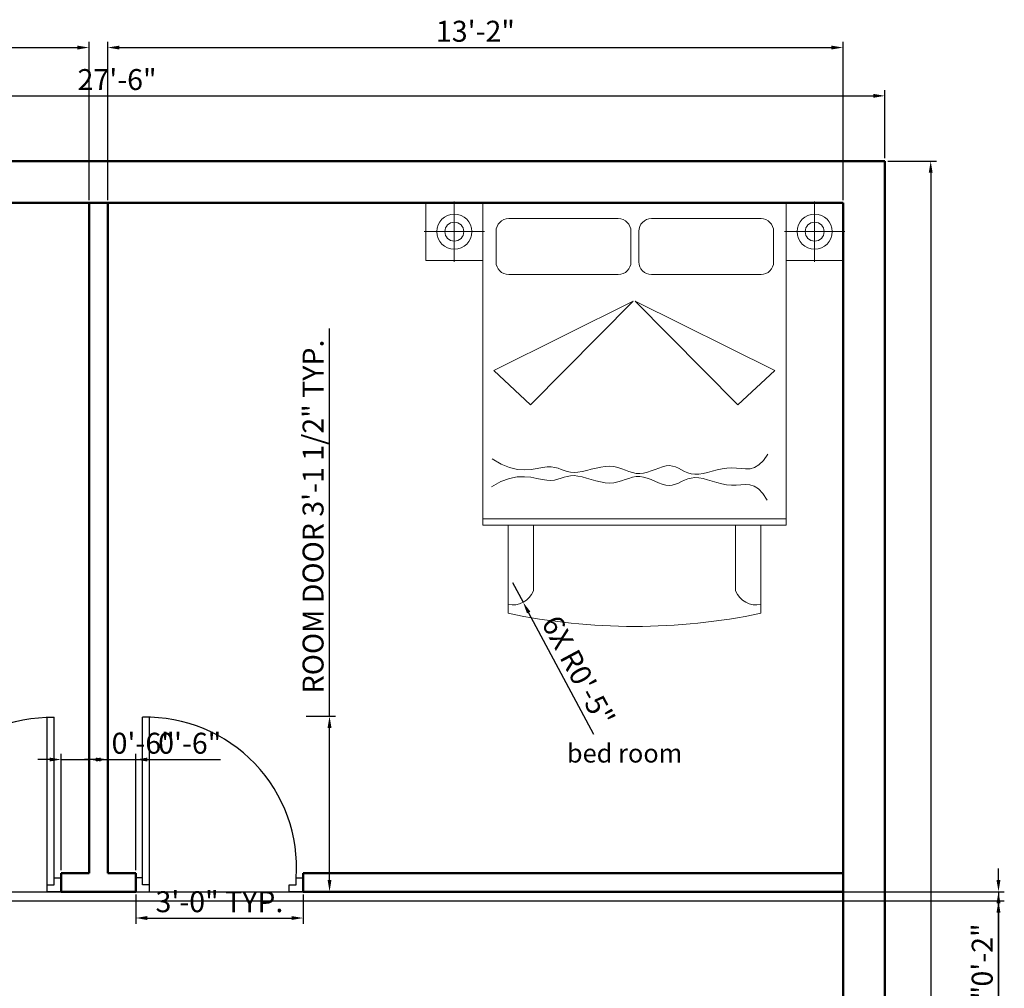
# Model space of a CAD drawing. Units: inches. Extents: x 1253 to 1645, y 2180 to 2698.
# Tile 5 of 5: x 1431 to 1643, y 2490 to 2698. Entities that reach past the tile are written whole.
import ezdxf

# ---------------------------------------------------------------- set-up
doc = ezdxf.new("R2010")
doc.units = ezdxf.units.IN
for name, color, linetype, lineweight in [('A-ANNO-DIMS', 2, 'Continuous', 18), ('A-AREA-IDEN', 7, 'Continuous', 25), ('A-DOOR', 4, 'Continuous', 25), ('A-FURN', 8, 'Continuous', 18), ('wall', 7, 'Continuous', 50)]:
    doc.layers.add(name, color=color, linetype=linetype, lineweight=lineweight)
doc.styles.get("Standard").update_dxf_attribs({"font": 'arial.ttf'})
doc.dimstyles.new('ISO-25', dxfattribs={"dimtxt": 4.5, "dimasz": 2.5, "dimexe": 1.25, "dimexo": 0.625, "dimtad": 1, "dimdec": 1, "dimlunit": 3, "dimtxsty": 'Standard', "dimcen": 4.5, "dimadec": 0, "dimazin": 0, "dimtfac": 1, "dimtdec": 1, "dimtmove": 0, "dimatfit": 3, "dimfxl": 1, "dimarcsym": 0})

# ---------------------------------------------------------------- blocks, each defined once
blk = doc.blocks.new('A$C4F543DC7')
for p, q in [((0.0134, 3.35, -0.1688), (3.3134, 3.35, -0.1688)), ((0.4634, 3.35, -0.1688), (0.0134, 3.35, -0.1688)), ((0.0134, 2.896, -0.1688), (0.0134, 3.35, -0.1688)), ((0.0134, 3.35, -0.1688), (0.0134, 2.896, -0.1688)), ((0.2381, 3.1233, -0.4388), (0.2381, 3.3614, -0.4388)), ((0.4634, 3.35, -0.1688), (0.4634, 0.8, -0.1688)), ((2.8634, 3.35, -0.1688), (0.4634, 3.35, -0.1688)), ((0.4634, 2.896, -0.1688), (0.4634, 3.35, -0.1688)), ((2.8634, 0.8, -0.1688), (2.8634, 3.35, -0.1688)), ((2.8634, 3.35, -0.1688), (3.3134, 3.35, -0.1688)), ((2.8634, 2.896, -0.1688), (2.8634, 3.35, -0.1688)), ((3.0888, 3.1233, -0.4388), (3.0888, 3.3614, -0.4388)), ((3.3134, 3.35, -0.1688), (3.3134, 2.896, -0.1688)), ((3.3134, 3.35, -0.1688), (3.3134, 2.896, -0.1688)), ((1.5354, 3.226, -0.1688), (0.6684, 3.226, -0.1688)), ((2.6644, 3.226, -0.1688), (1.7974, 3.226, -0.1688)), ((0.2381, 3.1233, -0.4388), (0, 3.1233, -0.4388)), ((0.2381, 3.1233, -0.4388), (0.4762, 3.1233, -0.4388)), ((0.2381, 3.1233, -0.4388), (0.2381, 2.8852, -0.4388)), ((0.5684, 3.126, -0.1688), (0.5684, 2.884, -0.1688)), ((1.6354, 2.884, -0.1688), (1.6354, 3.126, -0.1688)), ((1.6974, 3.126, -0.1688), (1.6974, 2.884, -0.1688)), ((2.7644, 2.884, -0.1688), (2.7644, 3.126, -0.1688)), ((3.0888, 3.1233, -0.4388), (2.8507, 3.1233, -0.4388)), ((3.0888, 3.1233, -0.4388), (3.0888, 2.8852, -0.4388)), ((3.0888, 3.1233, -0.4388), (3.3269, 3.1233, -0.4388)), ((0.4634, 2.896, -0.1688), (0.0134, 2.896, -0.1688)), ((0.0134, 2.896, -0.1688), (0.4634, 2.896, -0.1688)), ((0.4634, 0.8, -0.1688), (0.4634, 2.896, -0.1688)), ((2.8634, 2.896, -0.1688), (2.8634, 0.8, -0.1688)), ((3.3134, 2.896, -0.1688), (2.8634, 2.896, -0.1688)), ((3.3134, 2.896, -0.1688), (2.8634, 2.896, -0.1688)), ((0.6684, 2.784, -0.1688), (1.5354, 2.784, -0.1688)), ((1.7974, 2.784, -0.1688), (2.6644, 2.784, -0.1688)), ((1.6534, 2.573, -0.1688), (0.5504, 2.025, -0.1688)), ((0.8414, 1.752, -0.1688), (1.6534, 2.573, -0.1688)), ((2.4814, 1.752, -0.1688), (1.6694, 2.573, -0.1688)), ((1.6694, 2.573, -0.1688), (2.7724, 2.025, -0.1688)), ((0.5504, 2.025, -0.1688), (0.8414, 1.752, -0.1688)), ((2.7724, 2.025, -0.1688), (2.4814, 1.752, -0.1688)), ((0.5369, 1.3267, -0.1688), (0.6088, 1.2835, -0.1688)), ((2.683, 1.312, -0.1688), (2.7182, 1.3641, -0.1688)), ((0.6088, 1.2835, -0.1688), (0.6756, 1.2566, -0.1688)), ((0.6756, 1.2566, -0.1688), (0.7373, 1.2428, -0.1688)), ((0.8457, 1.242, -0.1688), (0.8925, 1.2489, -0.1688)), ((0.8925, 1.2489, -0.1688), (0.9345, 1.2564, -0.1688)), ((0.9345, 1.2564, -0.1688), (0.9718, 1.2615, -0.1688)), ((0.9718, 1.2615, -0.1688), (1.0044, 1.2617, -0.1688)), ((1.0044, 1.2617, -0.1688), (1.0334, 1.2578, -0.1688)), ((1.0334, 1.2578, -0.1688), (1.0597, 1.2509, -0.1688)), ((1.0597, 1.2509, -0.1688), (1.0842, 1.2424, -0.1688)), ((1.3218, 1.2441, -0.1688), (1.3591, 1.2533, -0.1688)), ((1.3591, 1.2533, -0.1688), (1.3963, 1.2612, -0.1688)), ((1.3963, 1.2612, -0.1688), (1.4328, 1.2664, -0.1688)), ((1.4328, 1.2664, -0.1688), (1.4679, 1.2677, -0.1688)), ((1.4679, 1.2677, -0.1688), (1.501, 1.2643, -0.1688)), ((1.501, 1.2643, -0.1688), (1.5324, 1.257, -0.1688)), ((1.5324, 1.257, -0.1688), (1.5624, 1.2473, -0.1688)), ((1.5624, 1.2473, -0.1688), (1.5915, 1.2365, -0.1688)), ((1.8258, 1.2417, -0.1688), (1.8557, 1.2531, -0.1688)), ((1.8557, 1.2531, -0.1688), (1.8849, 1.263, -0.1688)), ((1.8849, 1.263, -0.1688), (1.913, 1.2698, -0.1688)), ((1.913, 1.2698, -0.1688), (1.9397, 1.2722, -0.1688)), ((1.9397, 1.2722, -0.1688), (1.9649, 1.2692, -0.1688)), ((1.9649, 1.2692, -0.1688), (1.989, 1.2617, -0.1688)), ((1.989, 1.2617, -0.1688), (2.0124, 1.2512, -0.1688)), ((2.0124, 1.2512, -0.1688), (2.0359, 1.2391, -0.1688)), ((2.3173, 1.2378, -0.1688), (2.3558, 1.2465, -0.1688)), ((2.3558, 1.2465, -0.1688), (2.3944, 1.2527, -0.1688)), ((2.3944, 1.2527, -0.1688), (2.4325, 1.255, -0.1688)), ((2.4325, 1.255, -0.1688), (2.4698, 1.2529, -0.1688)), ((2.4698, 1.2529, -0.1688), (2.5064, 1.2488, -0.1688)), ((2.5064, 1.2488, -0.1688), (2.5423, 1.2459, -0.1688)), ((2.5423, 1.2459, -0.1688), (2.5777, 1.2476, -0.1688)), ((2.5777, 1.2476, -0.1688), (2.6129, 1.257, -0.1688)), ((2.6129, 1.257, -0.1688), (2.6479, 1.2774, -0.1688)), ((2.6479, 1.2774, -0.1688), (2.683, 1.312, -0.1688)), ((0.6067, 1.1458, -0.1688), (0.6743, 1.1706, -0.1688)), ((0.6743, 1.1706, -0.1688), (0.7364, 1.1825, -0.1688)), ((0.7364, 1.1825, -0.1688), (0.7931, 1.1846, -0.1688)), ((0.7373, 1.2428, -0.1688), (0.794, 1.239, -0.1688)), ((0.7931, 1.1846, -0.1688), (0.8447, 1.1799, -0.1688)), ((0.794, 1.239, -0.1688), (0.8457, 1.242, -0.1688)), ((0.8447, 1.1799, -0.1688), (0.8913, 1.1716, -0.1688)), ((0.8913, 1.1716, -0.1688), (0.9331, 1.1628, -0.1688)), ((1.0583, 1.1642, -0.1688), (1.0831, 1.172, -0.1688)), ((1.0831, 1.172, -0.1688), (1.1072, 1.18, -0.1688)), ((1.0842, 1.2424, -0.1688), (1.1081, 1.2336, -0.1688)), ((1.1072, 1.18, -0.1688), (1.1316, 1.1872, -0.1688)), ((1.1081, 1.2336, -0.1688), (1.1322, 1.2257, -0.1688)), ((1.1316, 1.1872, -0.1688), (1.1573, 1.192, -0.1688)), ((1.1322, 1.2257, -0.1688), (1.1577, 1.2201, -0.1688)), ((1.1573, 1.192, -0.1688), (1.1851, 1.1932, -0.1688)), ((1.1577, 1.2201, -0.1688), (1.1855, 1.218, -0.1688)), ((1.1851, 1.1932, -0.1688), (1.2158, 1.1898, -0.1688)), ((1.1855, 1.218, -0.1688), (1.2163, 1.2204, -0.1688)), ((1.2158, 1.1898, -0.1688), (1.2491, 1.1828, -0.1688)), ((1.2163, 1.2204, -0.1688), (1.2498, 1.2264, -0.1688)), ((1.2491, 1.1828, -0.1688), (1.2842, 1.1734, -0.1688)), ((1.2498, 1.2264, -0.1688), (1.2852, 1.2347, -0.1688)), ((1.2842, 1.1734, -0.1688), (1.3206, 1.1629, -0.1688)), ((1.2852, 1.2347, -0.1688), (1.3218, 1.2441, -0.1688)), ((1.5903, 1.1619, -0.1688), (1.6191, 1.1716, -0.1688)), ((1.5915, 1.2365, -0.1688), (1.6199, 1.2259, -0.1688)), ((1.6191, 1.1716, -0.1688), (1.6475, 1.1797, -0.1688)), ((1.6199, 1.2259, -0.1688), (1.6481, 1.2169, -0.1688)), ((1.6475, 1.1797, -0.1688), (1.676, 1.1849, -0.1688)), ((1.6481, 1.2169, -0.1688), (1.6765, 1.2108, -0.1688)), ((1.676, 1.1849, -0.1688), (1.7049, 1.1858, -0.1688)), ((1.6765, 1.2108, -0.1688), (1.7053, 1.209, -0.1688)), ((1.7049, 1.1858, -0.1688), (1.7344, 1.1816, -0.1688)), ((1.7053, 1.209, -0.1688), (1.7349, 1.2124, -0.1688)), ((1.7344, 1.1816, -0.1688), (1.7643, 1.1731, -0.1688)), ((1.7349, 1.2124, -0.1688), (1.7651, 1.2199, -0.1688)), ((1.7643, 1.1731, -0.1688), (1.7944, 1.1619, -0.1688)), ((1.7651, 1.2199, -0.1688), (1.7955, 1.2301, -0.1688)), ((1.7955, 1.2301, -0.1688), (1.8258, 1.2417, -0.1688)), ((2.0359, 1.2391, -0.1688), (2.0599, 1.2269, -0.1688)), ((2.0599, 1.2269, -0.1688), (2.0849, 1.216, -0.1688)), ((2.0842, 1.167, -0.1688), (2.1112, 1.1743, -0.1688)), ((2.0849, 1.216, -0.1688), (2.1117, 1.2077, -0.1688)), ((2.1112, 1.1743, -0.1688), (2.1403, 1.1775, -0.1688)), ((2.1117, 1.2077, -0.1688), (2.1407, 1.2037, -0.1688)), ((2.1403, 1.1775, -0.1688), (2.1718, 1.1755, -0.1688)), ((2.1407, 1.2037, -0.1688), (2.1723, 1.2047, -0.1688)), ((2.1718, 1.1755, -0.1688), (2.2056, 1.1691, -0.1688)), ((2.1723, 1.2047, -0.1688), (2.2062, 1.21, -0.1688)), ((2.2056, 1.1691, -0.1688), (2.2411, 1.1598, -0.1688)), ((2.2062, 1.21, -0.1688), (2.242, 1.2182, -0.1688)), ((2.242, 1.2182, -0.1688), (2.2791, 1.2279, -0.1688)), ((2.2791, 1.2279, -0.1688), (2.3173, 1.2378, -0.1688)), ((0.5334, 1.105, -0.1688), (0.6067, 1.1458, -0.1688)), ((0.9331, 1.1628, -0.1688), (0.9701, 1.1565, -0.1688)), ((0.9701, 1.1565, -0.1688), (1.0027, 1.1552, -0.1688)), ((1.0027, 1.1552, -0.1688), (1.0318, 1.1582, -0.1688)), ((1.0318, 1.1582, -0.1688), (1.0583, 1.1642, -0.1688)), ((1.3206, 1.1629, -0.1688), (1.3575, 1.1524, -0.1688)), ((1.3575, 1.1524, -0.1688), (1.3945, 1.1434, -0.1688)), ((1.3945, 1.1434, -0.1688), (1.4308, 1.1371, -0.1688)), ((1.4308, 1.1371, -0.1688), (1.4658, 1.1347, -0.1688)), ((1.4658, 1.1347, -0.1688), (1.499, 1.137, -0.1688)), ((1.499, 1.137, -0.1688), (1.5306, 1.1433, -0.1688)), ((1.5306, 1.1433, -0.1688), (1.5609, 1.152, -0.1688)), ((1.5609, 1.152, -0.1688), (1.5903, 1.1619, -0.1688)), ((1.7944, 1.1619, -0.1688), (1.8244, 1.1494, -0.1688)), ((1.8244, 1.1494, -0.1688), (1.8539, 1.137, -0.1688)), ((1.8539, 1.137, -0.1688), (1.8827, 1.1263, -0.1688)), ((1.8827, 1.1263, -0.1688), (1.9106, 1.1186, -0.1688)), ((1.9106, 1.1186, -0.1688), (1.9373, 1.1153, -0.1688)), ((1.9373, 1.1153, -0.1688), (1.9625, 1.1176, -0.1688)), ((1.9625, 1.1176, -0.1688), (1.9868, 1.1243, -0.1688)), ((1.9868, 1.1243, -0.1688), (2.0106, 1.134, -0.1688)), ((2.0106, 1.134, -0.1688), (2.0344, 1.1454, -0.1688)), ((2.0344, 1.1454, -0.1688), (2.0588, 1.1568, -0.1688)), ((2.0588, 1.1568, -0.1688), (2.0842, 1.167, -0.1688)), ((2.2411, 1.1598, -0.1688), (2.2779, 1.1489, -0.1688)), ((2.2779, 1.1489, -0.1688), (2.3157, 1.1379, -0.1688)), ((2.3157, 1.1379, -0.1688), (2.354, 1.1279, -0.1688)), ((2.354, 1.1279, -0.1688), (2.3923, 1.1205, -0.1688)), ((2.3923, 1.1205, -0.1688), (2.4304, 1.117, -0.1688)), ((2.4304, 1.117, -0.1688), (2.4677, 1.118, -0.1688)), ((2.4677, 1.118, -0.1688), (2.5043, 1.1209, -0.1688)), ((2.5043, 1.1209, -0.1688), (2.5403, 1.1226, -0.1688)), ((2.5403, 1.1226, -0.1688), (2.5757, 1.1199, -0.1688)), ((2.5757, 1.1199, -0.1688), (2.6106, 1.1094, -0.1688)), ((2.6106, 1.1094, -0.1688), (2.645, 1.0879, -0.1688)), ((2.645, 1.0879, -0.1688), (2.6789, 1.0522, -0.1688)), ((2.6789, 1.0522, -0.1688), (2.7124, 0.999, -0.1688)), ((0.4634, 0.85, -0.1688), (2.8634, 0.85, -0.1688)), ((0.4634, 0.8, -0.1688), (2.8634, 0.8, -0.1688)), ((0.6634, 0.8, -0.1688), (0.4634, 0.8, -0.1688)), ((0.6634, 0.8, -0.1688), (2.6634, 0.8, -0.1688)), ((0.6634, 0.104, -0.1688), (0.6634, 0.8, -0.1688)), ((0.6634, 0.104, -0.1688), (0.6634, 0.8, -0.1688)), ((0.8634, 0.281, -0.1688), (0.8634, 0.8, -0.1688)), ((2.4634, 0.8, -0.1688), (2.4634, 0.281, -0.1688)), ((2.8634, 0.8, -0.1688), (2.6634, 0.8, -0.1688)), ((2.6634, 0.8, -0.1688), (2.6634, 0.104, -0.1688)), ((2.6634, 0.8, -0.1688), (2.6634, 0.104, -0.1688))]:
    blk.add_line(p, q)
for centre, radius in [((0.2381, 3.1233, -0.4388), 0.139), ((0.2381, 3.1233, -0.4388), 0.075), ((3.0888, 3.1233, -0.4388), 0.139), ((3.0888, 3.1233, -0.4388), 0.075)]:
    blk.add_circle(centre, radius)
for centre, radius, start, end in [((0.6684, 3.126, -0.1688), 0.1, 90, 180), ((1.5354, 3.126, -0.1688), 0.1, 0, 90), ((1.7974, 3.126, -0.1688), 0.1, 90, 180), ((2.6644, 3.126, -0.1688), 0.1, 0, 90), ((0.6684, 2.884, -0.1688), 0.1, 180, 270), ((1.5354, 2.884, -0.1688), 0.1, 270, 0), ((1.7974, 2.884, -0.1688), 0.1, 180, 270), ((2.6644, 2.884, -0.1688), 0.1, 270, 0), ((0.6994, 0.3472, -0.1688), 0.1769, 258.2616, 338.03196), ((2.6275, 0.3472, -0.1688), 0.1769, 201.96804, 281.7384), ((1.6634, 4.8597, -0.1688), 4.8597, 258.12517, 281.87483), ((1.6634, 4.8597, -0.1688), 4.8597, 258.12517, 281.87483)]:
    blk.add_arc(centre, radius, start, end)
blk = doc.blocks.new('*D13')
at = {"layer": 'A-ANNO-DIMS', "color": 0, "lineweight": -2, "transparency": 16777216}
for p, q in [((1286.94, 2667.97), (1286.94, 2682.62)), ((1289.44, 2681.37), (1614.44, 2681.37)), ((1616.94, 2667.97), (1616.94, 2682.62))]:
    blk.add_line(p, q, dxfattribs=at)
at = {"layer": 'A-ANNO-DIMS', "color": 0, "transparency": 16777216}
for points in [[(1289.44, 2681.79), (1289.44, 2680.95), (1286.94, 2681.37)], [(1614.44, 2681.79), (1614.44, 2680.95), (1616.94, 2681.37)]]:
    blk.add_solid(points, dxfattribs=at)
at = {"layer": 'Defpoints', "color": 0, "transparency": 16777216}
for p in [(1616.94, 2681.37), (1286.94, 2667.35), (1616.94, 2667.35)]:
    blk.add_point(p, dxfattribs=at)
at = {"layer": 'A-ANNO-DIMS', "color": 0, "transparency": 16777216, "insert": (1451.94, 2684.29), "char_height": 4.5, "attachment_point": 5}
blk.add_mtext('27\'-6"', dxfattribs=at)
blk = doc.blocks.new('*D14')
at = {"layer": 'A-ANNO-DIMS', "color": 0, "lineweight": -2, "transparency": 16777216}
for p, q in [((1617.57, 2667.35), (1628.02, 2667.35)), ((1626.77, 2664.85), (1626.77, 2207.85)), ((1617.57, 2205.35), (1628.02, 2205.35))]:
    blk.add_line(p, q, dxfattribs=at)
at = {"layer": 'A-ANNO-DIMS', "color": 0, "transparency": 16777216}
for points in [[(1626.36, 2664.85), (1627.19, 2664.85), (1626.77, 2667.35)], [(1626.36, 2207.85), (1627.19, 2207.85), (1626.77, 2205.35)]]:
    blk.add_solid(points, dxfattribs=at)
at = {"layer": 'Defpoints', "color": 0, "transparency": 16777216}
for p in [(1616.94, 2667.35), (1616.94, 2205.35), (1626.77, 2205.35)]:
    blk.add_point(p, dxfattribs=at)
at = {"layer": 'A-ANNO-DIMS', "color": 0, "transparency": 16777216, "insert": (1623.85, 2436.35), "char_height": 4.5, "attachment_point": 5, "rotation": 90}
blk.add_mtext('38\'-6"', dxfattribs=at)
blk = doc.blocks.new('DOOR-SWING-36IN')
for p, q in [((1.5, 1.5), (1.5, 37.5)), ((3, 1.5), (3, 37.5)), ((0, 3), (0, 0)), ((1.5, 3), (0, 3)), ((1.5, 1.5), (1.5, 3)), ((34.5, 1.5), (34.5, 3)), ((34.5, 3), (36, 3)), ((36, 3), (36, 0)), ((3, 1.5), (1.5, 1.5)), ((3, 0), (3, 1.5)), ((33, 0), (33, 1.5)), ((33, 1.5), (34.5, 1.5)), ((0, 0), (3, 0)), ((36, 0), (33, 0))]:
    blk.add_line(p, q)
blk.add_arc((2.25, 5.18), 32.32, 356.1244, 91.3295)
blk = doc.blocks.new('*D16')
at = {"layer": 'A-ANNO-DIMS', "color": 0, "lineweight": -2, "transparency": 16777216}
for p, q in [((1497.6, 2548.06), (1497.6, 2631.4)), ((1492.57, 2548.06), (1498.85, 2548.06)), ((1497.6, 2512.85), (1497.6, 2545.56)), ((1492.57, 2510.35), (1498.85, 2510.35))]:
    blk.add_line(p, q, dxfattribs=at)
at = {"layer": 'A-ANNO-DIMS', "color": 0, "transparency": 16777216}
for points in [[(1497.18, 2545.56), (1498.01, 2545.56), (1497.6, 2548.06)], [(1497.18, 2512.85), (1498.01, 2512.85), (1497.6, 2510.35)]]:
    blk.add_solid(points, dxfattribs=at)
at = {"layer": 'Defpoints', "color": 0, "transparency": 16777216}
for p in [(1491.94, 2548.06), (1497.6, 2548.06), (1491.94, 2510.35)]:
    blk.add_point(p, dxfattribs=at)
at = {"layer": 'A-ANNO-DIMS', "color": 0, "transparency": 16777216, "insert": (1494.64, 2590.98), "char_height": 4.5, "attachment_point": 5, "rotation": 90}
blk.add_mtext('ROOM DOOR 3\'-1 1/2" TYP.', dxfattribs=at)
blk = doc.blocks.new('*D17')
at = {"layer": 'A-ANNO-DIMS', "color": 0, "lineweight": -2, "transparency": 16777216}
for p, q in [((1455.94, 2509.72), (1455.94, 2503.44)), ((1491.94, 2509.72), (1491.94, 2503.44)), ((1458.44, 2504.69), (1489.44, 2504.69))]:
    blk.add_line(p, q, dxfattribs=at)
at = {"layer": 'A-ANNO-DIMS', "color": 0, "transparency": 16777216}
for points in [[(1458.44, 2505.11), (1458.44, 2504.27), (1455.94, 2504.69)], [(1489.44, 2505.11), (1489.44, 2504.27), (1491.94, 2504.69)]]:
    blk.add_solid(points, dxfattribs=at)
at = {"layer": 'Defpoints', "color": 0, "transparency": 16777216}
for p in [(1455.94, 2510.35), (1491.94, 2510.35), (1491.94, 2504.69)]:
    blk.add_point(p, dxfattribs=at)
at = {"layer": 'A-ANNO-DIMS', "color": 0, "transparency": 16777216, "insert": (1473.94, 2507.61), "char_height": 4.5, "attachment_point": 5}
blk.add_mtext('3\'-0" TYP.', dxfattribs=at)
blk = doc.blocks.new('*D28')
at = {"layer": 'A-ANNO-DIMS', "color": 0, "lineweight": -2, "transparency": 16777216}
for p, q in [((1295.94, 2658.97), (1295.94, 2693)), ((1298.44, 2691.75), (1443.44, 2691.75)), ((1445.94, 2658.97), (1445.94, 2693))]:
    blk.add_line(p, q, dxfattribs=at)
at = {"layer": 'A-ANNO-DIMS', "color": 0, "transparency": 16777216}
for points in [[(1298.44, 2692.16), (1298.44, 2691.33), (1295.94, 2691.75)], [(1443.44, 2692.16), (1443.44, 2691.33), (1445.94, 2691.75)]]:
    blk.add_solid(points, dxfattribs=at)
at = {"layer": 'Defpoints', "color": 0, "transparency": 16777216}
for p in [(1445.94, 2691.75), (1295.94, 2658.35), (1445.94, 2658.35)]:
    blk.add_point(p, dxfattribs=at)
at = {"layer": 'A-ANNO-DIMS', "color": 0, "transparency": 16777216, "insert": (1370.94, 2694.67), "char_height": 4.5, "attachment_point": 5}
blk.add_mtext('12\'-6"', dxfattribs=at)
blk = doc.blocks.new('*D29')
at = {"layer": 'A-ANNO-DIMS', "color": 0, "lineweight": -2, "transparency": 16777216}
for p, q in [((1449.94, 2658.97), (1449.94, 2693)), ((1452.44, 2691.75), (1605.44, 2691.75)), ((1607.94, 2658.97), (1607.94, 2693))]:
    blk.add_line(p, q, dxfattribs=at)
at = {"layer": 'A-ANNO-DIMS', "color": 0, "transparency": 16777216}
for points in [[(1452.44, 2692.16), (1452.44, 2691.33), (1449.94, 2691.75)], [(1605.44, 2692.16), (1605.44, 2691.33), (1607.94, 2691.75)]]:
    blk.add_solid(points, dxfattribs=at)
at = {"layer": 'Defpoints', "color": 0, "transparency": 16777216}
for p in [(1607.94, 2691.75), (1449.94, 2658.35), (1607.94, 2658.35)]:
    blk.add_point(p, dxfattribs=at)
at = {"layer": 'A-ANNO-DIMS', "color": 0, "transparency": 16777216, "insert": (1528.94, 2694.67), "char_height": 4.5, "attachment_point": 5}
blk.add_mtext('13\'-2"', dxfattribs=at)
blk = doc.blocks.new('*D31')
at = {"layer": 'A-ANNO-DIMS', "color": 0, "lineweight": -2, "transparency": 16777216}
for p, q in [((1386.57, 2510.35), (1642.59, 2510.35)), ((1641.34, 2507.85), (1641.34, 2458.85)), ((1386.57, 2456.35), (1642.59, 2456.35))]:
    blk.add_line(p, q, dxfattribs=at)
at = {"layer": 'A-ANNO-DIMS', "color": 0, "transparency": 16777216}
for points in [[(1640.92, 2507.85), (1641.76, 2507.85), (1641.34, 2510.35)], [(1640.92, 2458.85), (1641.76, 2458.85), (1641.34, 2456.35)]]:
    blk.add_solid(points, dxfattribs=at)
at = {"layer": 'Defpoints', "color": 0, "transparency": 16777216}
for p in [(1385.94, 2510.35), (1385.94, 2456.35), (1641.34, 2456.35)]:
    blk.add_point(p, dxfattribs=at)
at = {"layer": 'A-ANNO-DIMS', "color": 0, "transparency": 16777216, "insert": (1638.42, 2483.35), "char_height": 4.5, "attachment_point": 5, "rotation": 90}
blk.add_mtext('4\'-6"', dxfattribs=at)
blk = doc.blocks.new('*D44')
at = {"layer": 'A-ANNO-DIMS', "color": 0, "lineweight": -2, "transparency": 16777216}
for p, q in [((1439.94, 2514.97), (1439.94, 2540)), ((1445.94, 2514.97), (1445.94, 2540)), ((1437.44, 2538.75), (1434.94, 2538.75)), ((1439.94, 2538.75), (1445.94, 2538.75)), ((1448.44, 2538.75), (1464.15, 2538.75))]:
    blk.add_line(p, q, dxfattribs=at)
at = {"layer": 'A-ANNO-DIMS', "color": 0, "transparency": 16777216}
for points in [[(1437.44, 2539.16), (1437.44, 2538.33), (1439.94, 2538.75)], [(1448.44, 2539.16), (1448.44, 2538.33), (1445.94, 2538.75)]]:
    blk.add_solid(points, dxfattribs=at)
at = {"layer": 'Defpoints', "color": 0, "transparency": 16777216}
for p in [(1445.94, 2538.75), (1439.94, 2514.35), (1445.94, 2514.35)]:
    blk.add_point(p, dxfattribs=at)
at = {"layer": 'A-ANNO-DIMS', "color": 0, "transparency": 16777216, "insert": (1457.55, 2541.67), "char_height": 4.5, "attachment_point": 5}
blk.add_mtext('0\'-6"', dxfattribs=at)
blk = doc.blocks.new('*D45')
at = {"layer": 'A-ANNO-DIMS', "color": 0, "lineweight": -2, "transparency": 16777216}
for p, q in [((1449.94, 2514.97), (1449.94, 2540)), ((1455.94, 2514.97), (1455.94, 2540)), ((1447.44, 2538.75), (1444.94, 2538.75)), ((1449.94, 2538.75), (1455.94, 2538.75)), ((1458.44, 2538.75), (1474.15, 2538.75))]:
    blk.add_line(p, q, dxfattribs=at)
at = {"layer": 'A-ANNO-DIMS', "color": 0, "transparency": 16777216}
for points in [[(1447.44, 2539.16), (1447.44, 2538.33), (1449.94, 2538.75)], [(1458.44, 2539.16), (1458.44, 2538.33), (1455.94, 2538.75)]]:
    blk.add_solid(points, dxfattribs=at)
at = {"layer": 'Defpoints', "color": 0, "transparency": 16777216}
for p in [(1455.94, 2538.75), (1449.94, 2514.35), (1455.94, 2514.35)]:
    blk.add_point(p, dxfattribs=at)
at = {"layer": 'A-ANNO-DIMS', "color": 0, "transparency": 16777216, "insert": (1467.55, 2541.67), "char_height": 4.5, "attachment_point": 5}
blk.add_mtext('0\'-6"', dxfattribs=at)
blk = doc.blocks.new('*D46')
at = {"layer": 'A-ANNO-DIMS', "color": 0, "lineweight": -2, "transparency": 16777216}
for p, q in [((1641.34, 2512.85), (1641.34, 2515.35)), ((1386.57, 2510.35), (1642.59, 2510.35)), ((1641.34, 2510.35), (1641.34, 2508.35)), ((1386.57, 2508.35), (1642.59, 2508.35)), ((1641.34, 2505.85), (1641.34, 2490.13))]:
    blk.add_line(p, q, dxfattribs=at)
at = {"layer": 'A-ANNO-DIMS', "color": 0, "transparency": 16777216}
for points in [[(1640.92, 2512.85), (1641.76, 2512.85), (1641.34, 2510.35)], [(1640.92, 2505.85), (1641.76, 2505.85), (1641.34, 2508.35)]]:
    blk.add_solid(points, dxfattribs=at)
at = {"layer": 'Defpoints', "color": 0, "transparency": 16777216}
for p in [(1385.94, 2510.35), (1385.94, 2508.35), (1641.34, 2508.35)]:
    blk.add_point(p, dxfattribs=at)
at = {"layer": 'A-ANNO-DIMS', "color": 0, "transparency": 16777216, "insert": (1638.42, 2496.74), "char_height": 4.5, "attachment_point": 5, "rotation": 90}
blk.add_mtext('0\'-2"', dxfattribs=at)
blk = doc.blocks.new('*D59')
at = {"layer": 'A-ANNO-DIMS', "color": 0, "lineweight": -2, "transparency": 16777216}
for p, q in [((1608.57, 2510.35), (1642.59, 2510.35)), ((1641.34, 2365.85), (1641.34, 2507.85)), ((1608.57, 2363.35), (1642.59, 2363.35))]:
    blk.add_line(p, q, dxfattribs=at)
at = {"layer": 'A-ANNO-DIMS', "color": 0, "transparency": 16777216}
for points in [[(1640.92, 2507.85), (1641.76, 2507.85), (1641.34, 2510.35)], [(1640.92, 2365.85), (1641.76, 2365.85), (1641.34, 2363.35)]]:
    blk.add_solid(points, dxfattribs=at)
at = {"layer": 'Defpoints', "color": 0, "transparency": 16777216}
for p in [(1607.94, 2510.35), (1641.34, 2510.35), (1607.94, 2363.35)]:
    blk.add_point(p, dxfattribs=at)
at = {"layer": 'A-ANNO-DIMS', "color": 0, "transparency": 16777216, "insert": (1638.42, 2436.85), "char_height": 4.5, "attachment_point": 5, "rotation": 90}
blk.add_mtext('12\'-3"', dxfattribs=at)
blk = doc.blocks.new('*D63')
at = {"layer": 'A-ANNO-DIMS', "color": 0, "lineweight": -2, "transparency": 16777216}
for p, q in [((1536.94, 2576.78), (1539.2, 2572.54)), ((1554.4, 2544.14), (1540.38, 2570.34))]:
    blk.add_line(p, q, dxfattribs=at)
at = {"layer": 'A-ANNO-DIMS', "color": 0, "transparency": 16777216}
blk.add_solid([(1540.75, 2570.54), (1540.02, 2570.14), (1539.2, 2572.54)], dxfattribs=at)
at = {"layer": 'Defpoints', "color": 0, "transparency": 16777216}
for p in [(1536.94, 2576.78), (1539.2, 2572.54)]:
    blk.add_point(p, dxfattribs=at)
at = {"layer": 'A-ANNO-DIMS', "color": 0, "transparency": 16777216, "insert": (1550.56, 2557.52), "char_height": 4.5, "attachment_point": 5, "rotation": 298.1516}
blk.add_mtext('6X R0\'-5"', dxfattribs=at)

msp = doc.modelspace()

# ---------------------------------------------------------------- linework, layer by layer
at = {"layer": 'wall'}
for p, q in [((1616.94, 2667.35), (1286.94, 2667.35)), ((1616.94, 2205.35), (1616.94, 2667.35)), ((1607.94, 2658.35), (1295.94, 2658.35)), ((1445.94, 2658.35), (1445.94, 2514.35)), ((1449.94, 2658.35), (1449.94, 2514.35)), ((1607.94, 2214.35), (1607.94, 2658.35)), ((1445.94, 2514.35), (1439.94, 2514.35)), ((1439.94, 2514.35), (1439.94, 2510.35)), ((1455.94, 2514.35), (1449.94, 2514.35)), ((1455.94, 2514.35), (1455.94, 2510.35)), ((1607.94, 2514.35), (1491.94, 2514.35)), ((1491.94, 2514.35), (1491.94, 2510.35)), ((1455.94, 2510.35), (1439.94, 2510.35)), ((1607.94, 2510.35), (1491.94, 2510.35))]:
    msp.add_line(p, q, dxfattribs=at)

# ---------------------------------------------------------------- block references
at = {"layer": 'A-DOOR', "extrusion": (0, 0, -1), "zscale": -1}
msp.add_blockref('DOOR-SWING-36IN', (-1439.94, 2510.35), dxfattribs=at)
at = {"layer": 'A-DOOR'}
msp.add_blockref('DOOR-SWING-36IN', (1455.94, 2510.35), dxfattribs=at)
at = {"layer": 'A-FURN', "xscale": 27.16316877811709, "yscale": 27.16316877811709, "zscale": 27.16316877811709}
msp.add_blockref('A$C4F543DC7', (1517.94, 2567.35, 4.58), dxfattribs=at)

# ---------------------------------------------------------------- texts
at = {"layer": 'A-AREA-IDEN', "insert": (1548.6, 2542.1), "char_height": 4, "attachment_point": 1}
msp.add_mtext_dynamic_manual_height_columns('bed room', width=71.3777, gutter_width=12.5, heights=[0], dxfattribs=at)

# ---------------------------------------------------------------- dimensions: what is measured, and where the dimension line sits
at = {"layer": 'A-ANNO-DIMS'}
for base, p1, p2, override, picture, middle in [((1445.94, 2691.75), (1295.94, 2658.35), (1445.94, 2658.35), {"dimdec": 1, "dimlfac": 1, "dimrnd": 0, "dimzin": 1, "dimdsep": 46, "dimlunit": 4, "dimfrac": 2}, '*D28', (1370.94, 2694.67)), ((1607.94, 2691.75), (1449.94, 2658.35), (1607.94, 2658.35), {"dimdec": 1, "dimlfac": 1, "dimrnd": 0, "dimzin": 1, "dimdsep": 46, "dimlunit": 4, "dimfrac": 2}, '*D29', (1528.94, 2694.67)), ((1616.94, 2681.37), (1286.94, 2667.35), (1616.94, 2667.35), {"dimclrd": 0, "dimclre": 0, "dimclrt": 0}, '*D13', (1451.94, 2684.29)), ((1445.94, 2538.75), (1439.94, 2514.35), (1445.94, 2514.35), {"dimdec": 1, "dimlfac": 1, "dimrnd": 0, "dimzin": 1, "dimdsep": 46, "dimlunit": 4, "dimfrac": 2}, '*D44', (1457.55, 2541.67)), ((1455.94, 2538.75), (1449.94, 2514.35), (1455.94, 2514.35), {"dimdec": 1, "dimlfac": 1, "dimrnd": 0, "dimzin": 1, "dimdsep": 46, "dimlunit": 4, "dimfrac": 2}, '*D45', (1467.55, 2541.67))]:
    dim = msp.add_linear_dim(base=base, p1=p1, p2=p2, dimstyle='ISO-25', override=override, dxfattribs=at)
    dim.commit()
    dim.dimension.update_dxf_attribs({"geometry": picture, "text_midpoint": middle})
for base, p1, p2, override, picture, middle in [((1626.77, 2205.35), (1616.94, 2667.35), (1616.94, 2205.35), {"dimclrd": 0, "dimclre": 0, "dimclrt": 0}, '*D14', (1623.85, 2436.35)), ((1641.34, 2508.35), (1385.94, 2510.35), (1385.94, 2508.35), {"dimdec": 1, "dimlfac": 1, "dimrnd": 0, "dimzin": 1, "dimdsep": 46, "dimlunit": 4, "dimfrac": 2}, '*D46', (1638.42, 2496.74)), ((1641.34, 2456.35), (1385.94, 2510.35), (1385.94, 2456.35), {"dimdec": 1, "dimlfac": 1, "dimrnd": 0, "dimzin": 1, "dimdsep": 46, "dimlunit": 4, "dimfrac": 2}, '*D31', (1638.42, 2483.35)), ((1641.34, 2510.35), (1607.94, 2363.35), (1607.94, 2510.35), {"dimdec": 1, "dimlfac": 1, "dimrnd": 0, "dimzin": 1, "dimdsep": 46, "dimlunit": 4, "dimfrac": 2}, '*D59', (1638.42, 2436.85))]:
    dim = msp.add_linear_dim(base=base, p1=p1, p2=p2, angle=90, dimstyle='ISO-25', override=override, dxfattribs=at)
    dim.commit()
    dim.dimension.update_dxf_attribs({"geometry": picture, "text_midpoint": middle})
dim = msp.add_linear_dim(base=(1497.6, 2548.06), p1=(1491.94, 2510.35), p2=(1491.94, 2548.06), angle=90, text='ROOM DOOR <> TYP.', dimstyle='ISO-25', override={"dimdec": 1, "dimlfac": 1, "dimrnd": 0, "dimzin": 1, "dimdsep": 46, "dimlunit": 4, "dimfrac": 2}, dxfattribs=at)
dim.commit()
dim.dimension.update_dxf_attribs({"geometry": '*D16', "text_midpoint": (1494.64, 2590.98)})
dim = msp.add_radius_dim(center=(1536.94, 2576.78), mpoint=(1539.2, 2572.54), text='6X <>', dimstyle='ISO-25', override={"dimdec": 1, "dimlfac": 1, "dimrnd": 0, "dimzin": 1, "dimdsep": 46, "dimlunit": 4, "dimfrac": 2}, dxfattribs=at)
dim.commit()
dim.dimension.update_dxf_attribs({"geometry": '*D63', "text_midpoint": (1550.56, 2557.52)})
dim = msp.add_linear_dim(base=(1491.94, 2504.69), p1=(1455.94, 2510.35), p2=(1491.94, 2510.35), text='<> TYP.', dimstyle='ISO-25', override={"dimdec": 1, "dimlfac": 1, "dimrnd": 0, "dimzin": 1, "dimdsep": 46, "dimlunit": 4, "dimfrac": 2}, dxfattribs=at)
dim.commit()
dim.dimension.update_dxf_attribs({"geometry": '*D17', "text_midpoint": (1473.94, 2507.61)})

doc.saveas('drawing.dxf')
